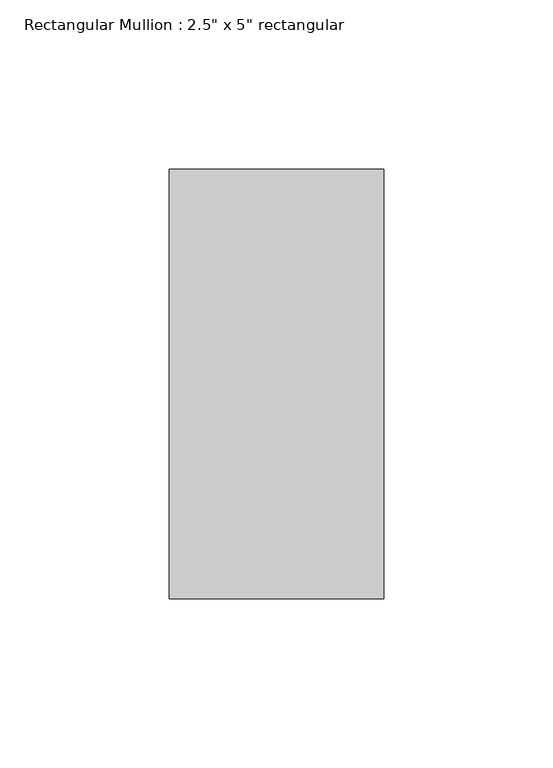
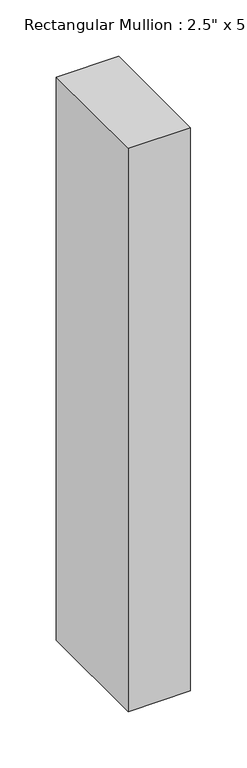
"""IFC4 building model written with IfcOpenShell, lengths in millimetres: member geometry."""

from ifc_helpers import new_model, si_unit, frame, origin, place, context, project, spatial, polyline, outline, extrude, source, transform, mapped, element, save


def member_ce3cb600(model_context):
    return source(origin(), model_context, "Body", "SweptSolid", [
        extrude(outline(polyline([(31.75, 63.5), (31.75, -63.5), (-31.75, -63.5), (-31.75, 63.5), (31.75, 63.5)])), frame((0.0, 0.0, -608.6004972), z_axis=(0.0, 0.0, 1.0), x_axis=(1.0, 0.0, 0.0)), (0.0, 0.0, 1.0), 608.6004972),
    ])


if __name__ == "__main__":
    model = new_model("IFC4")
    model_context = context("Model", 3, world=origin())
    ifc_project = project(units=[si_unit("LENGTHUNIT", "METRE", prefix="MILLI")], contexts=[model_context])
    site = spatial("IfcSite", under=ifc_project)
    building = spatial("IfcBuilding", under=site)
    placement = place(None, origin())
    member_shape = member_ce3cb600(model_context)
    element("IfcMember", 1, ObjectType="Rectangular Mullion : 2.5\" x 5\" rectangular", at=placement, inside=building, context=model_context, shape_type="MappedRepresentation", body=[
        mapped(member_shape, transform((0.0, 0.0, 0.0), x_axis=(1.0, 0.0, 0.0), y_axis=(0.0, 1.0, 0.0), z_axis=(0.0, 0.0, 1.0))),
    ])
    save(model, "model.ifc")

# Revit data of these elements
# Type "Rectangular Mullion : 2.5\" x 5\" rectangular"
#   built-in parameter 1007304 = 0.416667 (stored number, unit not read)
#   built-in parameter 1007301 = 0.104167 (stored number, unit not read)
#   built-in parameter 1007300 = 0.104167 (stored number, unit not read)
# Element 1 (IfcMember, "Rectangular Mullion : 2.5\" x 5\" rectangular")
#   Materials on its faces: "Aluminum"
# Materials
#   "Aluminum": class "Metal", colour RGB 247 247 247, transparency 0, Description = "Aluminum 6061", Cost = 0
